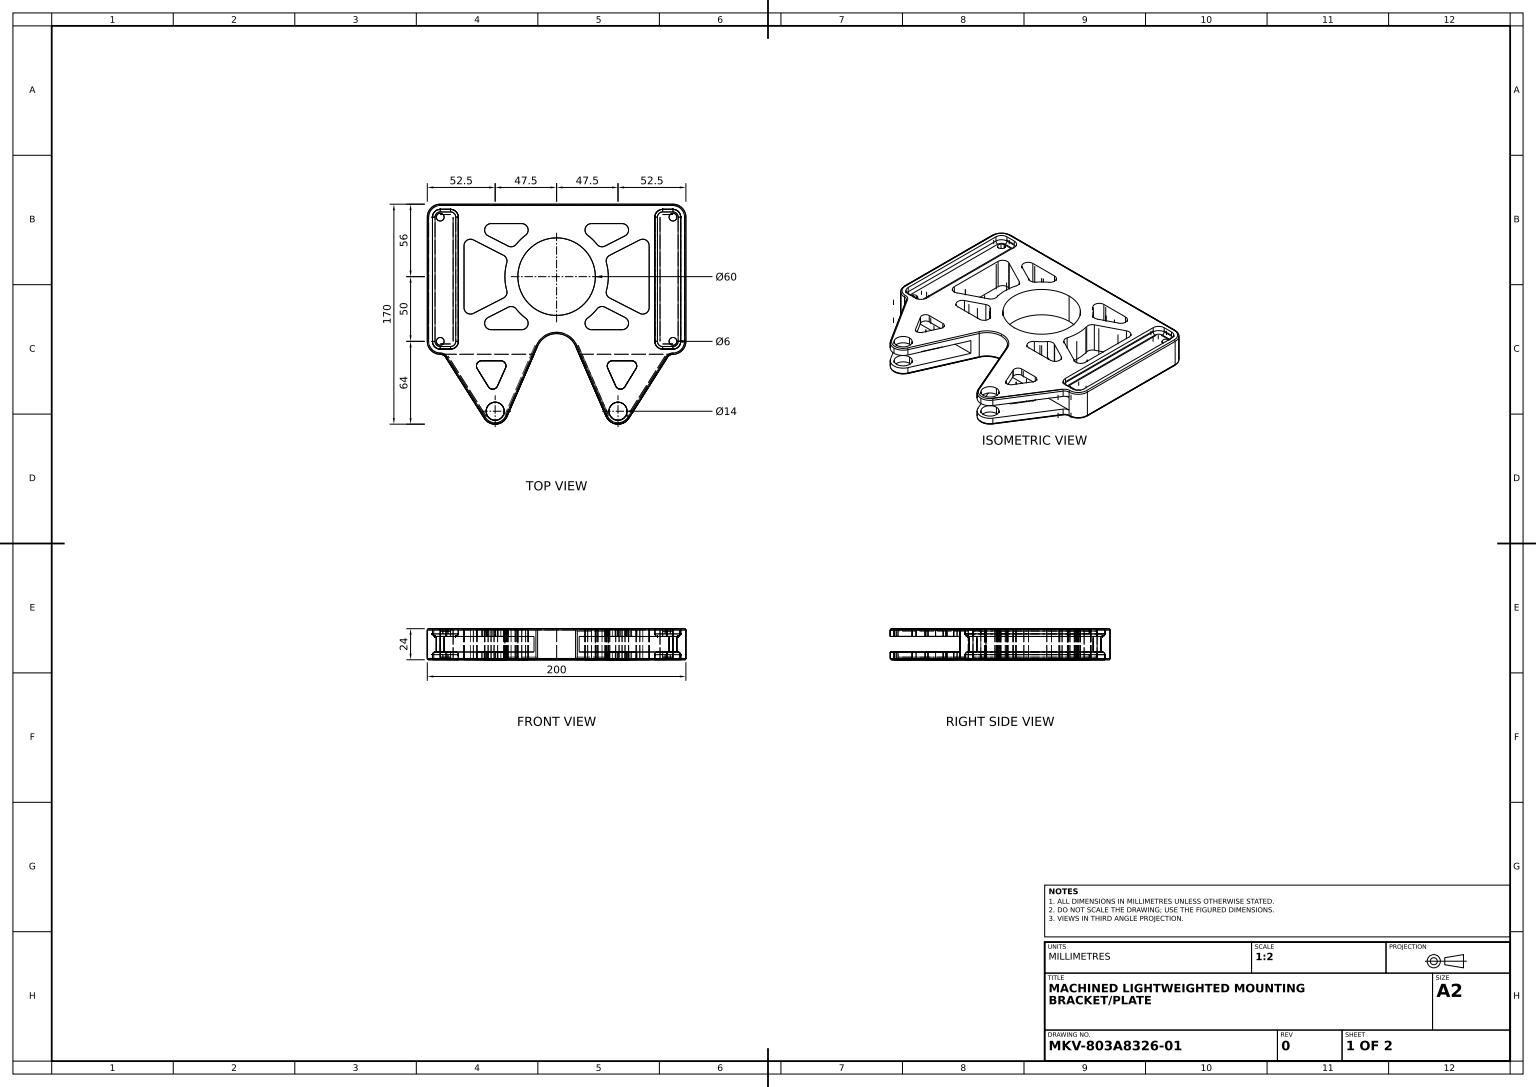
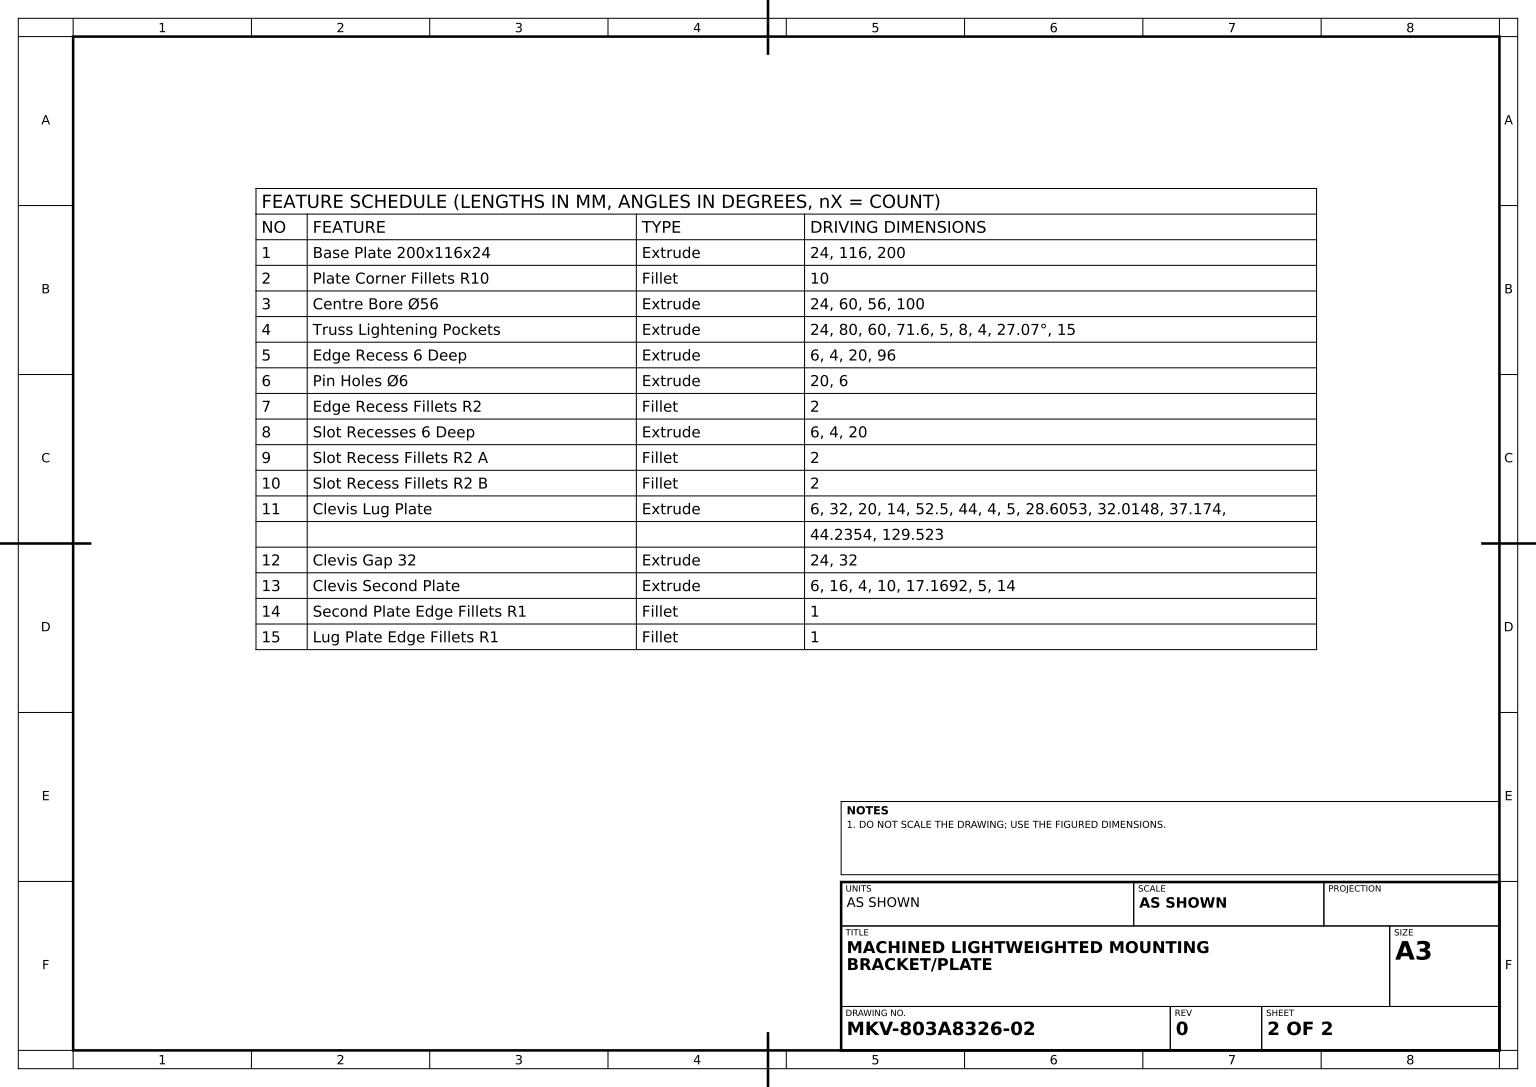
SolidWorks part; units mm, degrees
material "Plain Carbon Steel"
ref_plane "Front Plane" through (0, 0, 0) normal (0, 0, 1) x (1, 0, 0)
ref_plane "Top Plane" through (0, 0, 0) normal (0, 1, 0) x (1, 0, 0)
ref_plane "Right Plane" through (0, 0, 0) normal (1, 0, 0) x (0, 0, -1)
sketch "Base Plate Sketch" plane through (0, 0, 0) normal (0, 1, 0) x (1, 0, 0)
  line L1 (-100, -58) -> (100, -58)
  line L2 (-100, -58) -> (-100, 58)
  line L3 (-100, 58) -> (100, 58)
  line L4 (100, -58) -> (100, 58)
  line L5 (-100, -58) -> (100, 58) construction
  line L6 (-100, 58) -> (100, -58) construction
  point P0 (0, 0)
  dimension "D1" = 116
  dimension "D2" = 200
extrude "Base Plate 200x116x24" add sketch "Base Plate Sketch" along normal blind 24
fillet "Plate Corner Fillets R10" radius 10 4 edges at (-100, 12, -58) (100, 12, -58) (100, 12, 58) (-100, 12, 58)
sketch "Centre Bore Sketch" plane through (0, 24, 0) normal (0, 1, 0) x (1, 0, 0)
  line L0 (90, 58) -> (-90, 58) construction
  line L1 (-100, 48) -> (-100, -48) construction
  circle A0 centre (0, 2) radius 30
  dimension "D1" = 60
  dimension "D2" = 56
  dimension "D3" = 100
extrude "Centre Bore Ø56" cut sketch "Centre Bore Sketch" against normal blind 24
sketch "Truss Pocket Sketch" plane through (0, 24, 0) normal (0, 1, 0) x (1, 0, 0)
  line L0 (71.6, -21.9326) -> (71.6, 25.9326)
  line L3 (0, 2) -> (71.6, 2)
  line L5 (41.0804, 18.5045) -> (64.3244, 30.3848)
  line L6 (37.4395, 25.628) -> (52.9349, 33.5478)
  line L7 (41.0804, -14.5045) -> (64.3244, -26.3848)
  line L8 (0, 58) -> (0, -58)
  line L10 (50.6594, 43) -> (27, 43)
  line L12 (90, 58) -> (-90, 58) construction
  line L14 (-90, -58) -> (90, -58) construction
  line L15 (37.4395, -21.628) -> (52.9349, -29.5478)
  line L16 (50.6594, -39) -> (27, -39)
  line L17 (-50.6594, -39) -> (-27, -39)
  line L18 (-37.4395, -21.628) -> (-52.9349, -29.5478)
  line L19 (-41.0804, -14.5045) -> (-64.3244, -26.3848)
  line L20 (-71.6, -21.9326) -> (-71.6, 25.9326)
  line L21 (-41.0804, 18.5045) -> (-64.3244, 30.3848)
  line L22 (-37.4395, 25.628) -> (-52.9349, 33.5478)
  line L23 (-50.6594, 43) -> (-27, 43)
  circle A1 centre (0, 2) radius 30
  arc A2 (24, -30) -> (31.2569, -22.9601) centre (0, 2) ccw
  arc A3 (64.3244, 30.3848) -> (71.6, 25.9326) centre (66.6, 25.9326) cw
  arc A4 (41.0804, 18.5045) -> (38.5387, 12.7132) centre (43.356, 14.0523) ccw
  arc A5 (64.3244, -26.3848) -> (71.6, -21.9326) centre (66.6, -21.9326) ccw
  arc A6 (41.0804, -14.5045) -> (38.5387, -8.7132) centre (43.356, -10.0523) cw
  arc A7 (27, 43) -> (24, 34) centre (27, 38) ccw
  arc A8 (31.2569, 26.9601) -> (37.4395, 25.628) centre (35.164, 30.0801) ccw
  arc A9 (50.6594, 43) -> (52.9349, 33.5478) centre (50.6594, 38) cw
  arc A10 (31.2569, -22.9601) -> (37.4395, -21.628) centre (35.164, -26.0801) cw
  arc A11 (50.6594, -39) -> (52.9349, -29.5478) centre (50.6594, -34) ccw
  arc A12 (27, -39) -> (24, -30) centre (27, -34) cw
  arc A13 (31.2569, 26.9601) -> (24, 34) centre (0, 2) ccw
  arc A14 (38.5387, -8.7132) -> (38.5387, 12.7132) centre (0, 2) ccw
  arc A15 (-27, -39) -> (-24, -30) centre (-27, -34) ccw
  arc A16 (-50.6594, -39) -> (-52.9349, -29.5478) centre (-50.6594, -34) cw
  arc A17 (-31.2569, -22.9601) -> (-37.4395, -21.628) centre (-35.164, -26.0801) ccw
  arc A18 (-24, -30) -> (-31.2569, -22.9601) centre (0, 2) cw
  arc A19 (-64.3244, -26.3848) -> (-71.6, -21.9326) centre (-66.6, -21.9326) cw
  arc A20 (-41.0804, -14.5045) -> (-38.5387, -8.7132) centre (-43.356, -10.0523) ccw
  arc A21 (-64.3244, 30.3848) -> (-71.6, 25.9326) centre (-66.6, 25.9326) ccw
  arc A22 (-38.5387, -8.7132) -> (-38.5387, 12.7132) centre (0, 2) cw
  arc A23 (-41.0804, 18.5045) -> (-38.5387, 12.7132) centre (-43.356, 14.0523) cw
  arc A24 (-31.2569, 26.9601) -> (-37.4395, 25.628) centre (-35.164, 30.0801) cw
  arc A25 (-31.2569, 26.9601) -> (-24, 34) centre (0, 2) cw
  arc A26 (-50.6594, 43) -> (-52.9349, 33.5478) centre (-50.6594, 38) ccw
  arc A27 (-27, 43) -> (-24, 34) centre (-27, 38) cw
  point P11 (1.8204, -1.5617)
  point P13 (90, 48)
  point P15 (91.8204, 44.4383)
  point P16 (-1.8204, 5.5617)
  point P17 (88.1796, 51.5617)
  dimension "D1" = 80
  dimension "D2" = 60
  dimension "D6" = 5
  dimension "D7" = 5
  dimension "D9" = 5
  dimension "D10" = 5
  dimension "D11" = 5
  dimension "D3" = 71.6
  dimension "D4" = 8
  dimension "D5" = 4
  dimension "D8" = 27.072
  dimension "D12" = 15
extrude "Truss Lightening Pockets" cut sketch "Truss Pocket Sketch" against normal blind 24 contours A27 L23 A26 L22 A24 A25 | A23 L21 A21 L20 A19 L19 A20 A22 | A13 A8 L6 A9 L10 A7 | A14 L3 L0 A3 L5 A4 | A14 A6 L7 A5 L0 L3 | A12 L16 A11 L15 A10 A2 | A15 A18 A17 L18 A16 L17
sketch "Edge Recess Sketch" plane through (0, 24, 0) normal (0, 1, 0) x (1, 0, 0)
  line L0 (96, 48) -> (96, -48)
  line L1 (0, 58) -> (0, -58)
  line L2 (90, 58) -> (-90, 58) construction
  line L3 (76, 48) -> (76, -48)
  line L4 (90, 54) -> (-90, 54)
  line L5 (90, 54) -> (82, 54)
  line L6 (-90, -58) -> (90, -58) construction
  line L7 (-82, -54) -> (-90, -54)
  line L8 (-90, -54) -> (90, -54)
  line L9 (82, -54) -> (90, -54)
  line L10 (-76, 48) -> (-76, -48)
  line L11 (-96, 48) -> (-96, -48)
  line L12 (-90, 54) -> (-82, 54)
  arc A0 (-90, -54) -> (-96, -48) centre (-90, -48) cw
  arc A1 (-76, -48) -> (-82, -54) centre (-82, -48) cw
  arc A3 (90, 54) -> (96, 48) centre (90, 48) cw
  arc A4 (76, 48) -> (82, 54) centre (82, 48) cw
  arc A5 (76, -48) -> (82, -54) centre (82, -48) ccw
  arc A6 (90, -54) -> (96, -48) centre (90, -48) ccw
  arc A7 (-90, 54) -> (-96, 48) centre (-90, 48) ccw
  arc A8 (-76, 48) -> (-82, 54) centre (-82, 48) ccw
  dimension "D1" = 96
  dimension "D5" = 6
  dimension "D6" = 6
  dimension "D7" = 6
  dimension "D2" = 4
  dimension "D3" = 20
  dimension "D4" = 4
extrude "Edge Recess 6 Deep" cut sketch "Edge Recess Sketch" against normal blind 6 contours L9 A6 L0 A3 L5 A4 L3 A5 | L10 A8 L12 A7 L11 A0 L7 A1
sketch "Pin Hole Sketch" plane through (0, 18, 0) normal (0, 1, 0) x (1, 0, 0)
  circle A0 centre (90, 48) radius 3
  circle A1 centre (90, -48) radius 3
  circle A2 centre (-90, 48) radius 3
  circle A3 centre (-90, -48) radius 3
  dimension "D1" = 6
  dimension "D2" = 6
  dimension "D3" = 6
  dimension "D4" = 6
extrude "Pin Holes Ø6" cut sketch "Pin Hole Sketch" against normal blind 20
fillet "Edge Recess Fillets R2" radius 2 16 edges at (77.7574, 18, -52.2426) (86, 18, -54) (94.2426, 18, -52.2426) (96, 18, 0) (94.2426, 18, 52.2426) (86, 18, 54) (77.7574, 18, 52.2426) (-94.2426, 18, -52.2426) (-86, 18, -54) (-77.7574, 18, -52.2426) (-76, 18, 0) (-77.7574, 18, 52.2426) (-86, 18, 54) (-94.2426, 18, 52.2426) (76, 18, 0) (-96, 18, 0)
sketch "Slot Recess Sketch" plane through (0, 0, 0) normal (0, -1, 0) x (1, 0, 0)
  line L5 (-96, -48) -> (-96, 48)
  line L6 (-96, -48) -> (-96, 48)
  line L8 (-90, 54) -> (90, 54)
  line L9 (-90, 54) -> (-82, 54)
  line L11 (90, -54) -> (-90, -54)
  line L12 (90, -54) -> (82, -54)
  line L13 (-76, -48) -> (-76, 48)
  line L14 (96, 48) -> (96, -48)
  line L15 (96, 48) -> (96, -48)
  line L16 (76, 48) -> (76, -48)
  line L17 (82, 54) -> (90, 54)
  line L18 (-82, -54) -> (-90, -54)
  arc A0 (-96, 48) -> (-90, 54) centre (-90, 48) cw
  arc A1 (-96, -48) -> (-90, -54) centre (-90, -48) ccw
  arc A2 (90, -54) -> (96, -48) centre (90, -48) ccw
  arc A3 (90, 54) -> (96, 48) centre (90, 48) cw
  arc A4 (-82, 54) -> (-76, 48) centre (-82, 48) cw
  arc A5 (-76, -48) -> (-82, -54) centre (-82, -48) cw
  arc A6 (82, 54) -> (76, 48) centre (82, 48) ccw
  arc A7 (76, -48) -> (82, -54) centre (82, -48) ccw
  dimension "D5" = 20
  dimension "D7" = 6
  dimension "D8" = 6
  dimension "D9" = 6
  dimension "D10" = 6
  dimension "D1" = 4
  dimension "D2" = 4
  dimension "D3" = 4
  dimension "D4" = 4
  dimension "D6" = 20
extrude "Slot Recesses 6 Deep" cut sketch "Slot Recess Sketch" against normal blind 6
fillet "Slot Recess Fillets R2 A" radius 2 8 edges at (-94.2426, 6, 52.2426) (-86, 6, 54) (-77.7574, 6, 52.2426) (-76, 6, 0) (-77.7574, 6, -52.2426) (-86, 6, -54) (-94.2426, 6, -52.2426) (-96, 6, 0)
fillet "Slot Recess Fillets R2 B" radius 2 8 edges at (77.7574, 6, 52.2426) (86, 6, 54) (94.2426, 6, 52.2426) (96, 6, 0) (94.2426, 6, -52.2426) (86, 6, -54) (77.7574, 6, -52.2426) (76, 6, 0)
ref_plane "Clevis Lug Plane" through (0, 0, 0) normal (0, 1, 0) x (1, 0, 0)
sketch "Clevis Lug Plate Sketch" plane through (0, 0, 0) normal (0, 1, 0) x (1, 0, 0)
  line L0 (-90, -58) -> (90, -58) construction
  line L1 (-61.3947, -69.0917) -> (-52.826, -83.0589)
  line L2 (-85.7777, -60.3219) -> (-55.9446, -107.3563)
  line L3 (-38.3304, -105.9899) -> (-14.6713, -51.6162)
  line L4 (38.3304, -105.9899) -> (14.6713, -51.6162)
  line L5 (-100, 48) -> (-100, -48) construction
  line L6 (85.7777, -60.3219) -> (55.9446, -107.3563)
  line L7 (-45.7646, -82.5992) -> (-39.5228, -68.632)
  line L9 (-57.9852, -63) -> (-43.1747, -63)
  line L10 (-90, -58) -> (-17.449, -58)
  line L11 (45.7646, -82.5992) -> (39.5228, -68.632)
  line L12 (61.3947, -69.0917) -> (52.826, -83.0589)
  line L13 (57.9852, -63) -> (43.1747, -63)
  line L14 (17.449, -58) -> (90, -58)
  arc A0 (14.6713, -51.6162) -> (-14.6713, -51.6162) centre (0, -58) ccw
  arc A1 (-55.9446, -107.3563) -> (-38.3304, -105.9899) centre (-47.5, -102) ccw
  circle A2 centre (-47.5, -102) radius 7
  arc A3 (-90, -58) -> (-85.7777, -60.3219) centre (-90, -63) cw
  arc A4 (55.9446, -107.3563) -> (38.3304, -105.9899) centre (47.5, -102) cw
  circle A5 centre (47.5, -102) radius 7
  arc A6 (90, -58) -> (85.7777, -60.3219) centre (90, -63) ccw
  arc A7 (-52.826, -83.0589) -> (-45.7646, -82.5992) centre (-49.4165, -80.9672) ccw
  arc A8 (-57.9852, -63) -> (-61.3947, -69.0917) centre (-57.9852, -67) ccw
  arc A9 (-43.1747, -63) -> (-39.5228, -68.632) centre (-43.1747, -67) cw
  arc A10 (43.1747, -63) -> (39.5228, -68.632) centre (43.1747, -67) ccw
  arc A11 (52.826, -83.0589) -> (45.7646, -82.5992) centre (49.4165, -80.9672) cw
  arc A12 (57.9852, -63) -> (61.3947, -69.0917) centre (57.9852, -67) cw
  dimension "D1" = 32
  dimension "D4" = 20
  dimension "D5" = 14
  dimension "D2" = 4
  dimension "D3" = 4
  dimension "D9" = 4
  dimension "D8" = 5
  dimension "D6" = 44
  dimension "D7" = 52.5
  dimension "D10" = 28.6053
  dimension "D11" = 32.0148
  dimension "D12" = 37.174
  dimension "D13" = 44.2354
  dimension "D14" = 129.5228
extrude "Clevis Lug Plate" add sketch "Clevis Lug Plate Sketch" along normal blind 6 contours L10 A3 L2 A1 L3 A2 L9 A9 L7 A7 L1 A8 | A6 L14 L4 A4 L6 A5 L13 A12 L12 A11 L11 A10
sketch "Clevis Gap Sketch" plane through (0, 24, 0) normal (0, 1, 0) x (1, 0, 0)
  line L0 (-90, -58) -> (90, -58) construction
  line L1 (-17.449, -58) -> (-14.6713, -51.6162)
  line L2 (17.449, -58) -> (14.6713, -51.6162)
  line L3 (-17.449, -58) -> (17.449, -58)
  arc A0 (14.6713, -51.6162) -> (-14.6713, -51.6162) centre (0, -58) ccw
  dimension "D1" = 32
extrude "Clevis Gap 32" cut sketch "Clevis Gap Sketch" against normal blind 24
sketch "Clevis Second Plate Sketch" plane through (0, 24, 0) normal (0, 1, 0) x (1, 0, 0)
  line L0 (-90, -58) -> (-17.449, -58)
  line L1 (-85.7777, -60.3219) -> (-55.9446, -107.3563)
  line L2 (-38.3304, -105.9899) -> (-14.6713, -51.6162)
  line L3 (14.6713, -51.6162) -> (38.3304, -105.9899)
  line L4 (55.9446, -107.3563) -> (85.7777, -60.3219)
  line L5 (17.449, -58) -> (90, -58)
  line L6 (-57.9852, -63) -> (-43.1747, -63)
  line L7 (-39.5228, -68.632) -> (-45.7646, -82.5992)
  line L8 (-61.3947, -69.0917) -> (-52.3507, -83.6857)
  line L9 (52.826, -83.0589) -> (61.3947, -69.0917)
  line L10 (57.9852, -63) -> (43.1747, -63)
  line L11 (39.5228, -68.632) -> (45.7646, -82.5992)
  arc A0 (-14.6713, -51.6162) -> (14.6713, -51.6162) centre (0, -58) cw
  arc A1 (-90, -58) -> (-85.7777, -60.3219) centre (-90, -63) cw
  arc A2 (90, -58) -> (85.7777, -60.3219) centre (90, -63) ccw
  arc A3 (38.3304, -105.9899) -> (55.9446, -107.3563) centre (47.5, -102) ccw
  arc A4 (-55.9446, -107.3563) -> (-38.3304, -105.9899) centre (-47.5, -102) ccw
  arc A5 (-57.9852, -63) -> (-61.3947, -69.0917) centre (-57.9852, -67) ccw
  arc A6 (-43.1747, -63) -> (-39.5228, -68.632) centre (-43.1747, -67) cw
  arc A7 (-52.3507, -83.6857) -> (-45.7646, -82.5992) centre (-49.4165, -80.9672) ccw
  arc A8 (-52.826, -83.0589) -> (-45.7646, -82.5992) centre (-49.4165, -80.9672) ccw construction
  arc A9 (39.5228, -68.632) -> (43.1747, -63) centre (43.1747, -67) cw
  arc A10 (57.9852, -63) -> (61.3947, -69.0917) centre (57.9852, -67) cw
  arc A11 (45.7646, -82.5992) -> (52.826, -83.0589) centre (49.4165, -80.9672) ccw
  circle A12 centre (-47.5, -102) radius 7
  circle A14 centre (47.5, -102) radius 7
  dimension "D1" = 16
  dimension "D2" = 4
  dimension "D3" = 10
  dimension "D4" = 4
  dimension "D6" = 5
  dimension "D7" = 14
  dimension "D8" = 14
  dimension "D5" = 17.1692
extrude "Clevis Second Plate" add sketch "Clevis Second Plate Sketch" against normal blind 6 contours L1 A4 L2 L0 A1 A12 A7 L8 A5 L6 A6 L7 | L3 A3 L4 A2 L5 A14 A11 L11 A9 L10 A10 L9
fillet "Second Plate Edge Fillets R1" radius 1 16 edges at (0, 24, 42) (26.5009, 24, 78.803) (46.7266, 24, 111.97) (70.8611, 24, 83.8391) (87.5907, 24, 58.6188) (97.0711, 24, 55.0711) (100, 24, 0) (97.0711, 24, -55.0711) (0, 24, -58) (-97.0711, 24, -55.0711) (-100, 24, 0) (-97.0711, 24, 55.0711) (-87.5907, 24, 58.6188) (-70.8611, 24, 83.8391) (-46.7266, 24, 111.97) (-26.5009, 24, 78.803)
fillet "Lug Plate Edge Fillets R1" radius 1 16 edges at (-46.7266, 0, 111.97) (-70.8611, 0, 83.8391) (-87.5907, 0, 58.6188) (-97.0711, 0, 55.0711) (-100, 0, 0) (-97.0711, 0, -55.0711) (0, 0, -58) (97.0711, 0, -55.0711) (100, 0, 0) (97.0711, 0, 55.0711) (87.5907, 0, 58.6188) (70.8611, 0, 83.8391) (46.7266, 0, 111.97) (26.5009, 0, 78.803) (0, 0, 42) (-26.5009, 0, 78.803)
